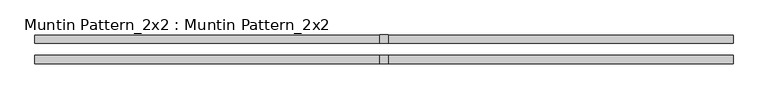
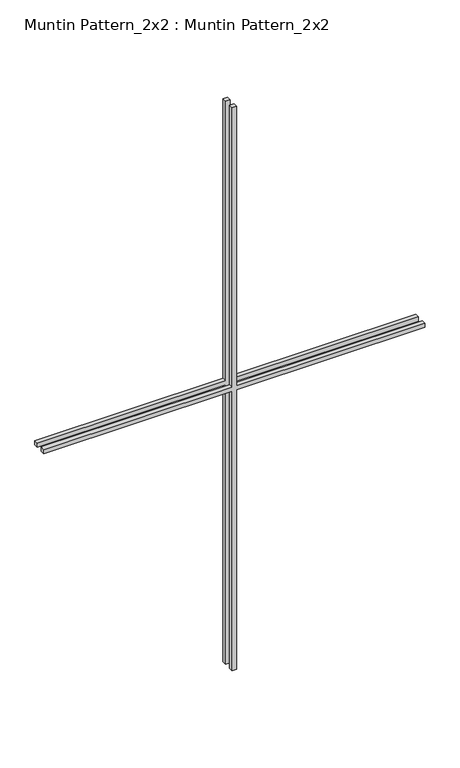
"""IFC4 building model written with IfcOpenShell, lengths in millimetres: proxy geometry, Muntin Pattern_2x2 : Muntin Pattern_2x2."""

from ifc_helpers import new_model, si_unit, frame, origin, place, context, project, spatial, polyline, outline, extrude, source, transform, mapped, element, save


def muntin_pattern_2x2_muntin_pattern_2x2_bb8d4d84(model_context):
    return source(origin(), model_context, "Body", "SweptSolid", [
        extrude(outline(polyline([(850.9, -6.35), (850.9, -541.3375), (838.2, -541.3375), (838.2, -6.35), (0.0, -6.35), (0.0, 6.35), (838.2, 6.35), (838.2, 541.3375), (850.9, 541.3375), (850.9, 6.35), (1689.1, 6.35), (1689.1, -6.35), (850.9, -6.35)])), frame((0.0, 9.525, 0.0), z_axis=(0.0, 1.0, 0.0), x_axis=(0.0, 0.0, 1.0)), (0.0, 0.0, 1.0), 12.7),
        extrude(outline(polyline([(850.9, -6.35), (850.9, -541.3375), (838.2, -541.3375), (838.2, -6.35), (0.0, -6.35), (0.0, 6.35), (838.2, 6.35), (838.2, 541.3375), (850.9, 541.3375), (850.9, 6.35), (1689.1, 6.35), (1689.1, -6.35), (850.9, -6.35)])), frame((0.0, -22.225, 0.0), z_axis=(0.0, 1.0, 0.0), x_axis=(0.0, 0.0, 1.0)), (0.0, 0.0, 1.0), 12.7),
    ])


if __name__ == "__main__":
    model = new_model("IFC4")
    model_context = context("Model", 3, world=origin())
    ifc_project = project(units=[si_unit("LENGTHUNIT", "METRE", prefix="MILLI")], contexts=[model_context])
    site = spatial("IfcSite", under=ifc_project)
    building = spatial("IfcBuilding", under=site)
    placement = place(None, origin())
    muntin_pattern_2x2_muntin_pattern_2x2_shape = muntin_pattern_2x2_muntin_pattern_2x2_bb8d4d84(model_context)
    element("IfcBuildingElementProxy", 1, Name="Muntin Pattern_2x2 : Muntin Pattern_2x2", ObjectType="Muntin Pattern_2x2 : Muntin Pattern_2x2", at=placement, inside=building, context=model_context, shape_type="MappedRepresentation", body=[
        mapped(muntin_pattern_2x2_muntin_pattern_2x2_shape, transform((0.0, 0.0, 0.0), x_axis=(1.0, 0.0, 0.0), y_axis=(0.0, 1.0, 0.0), z_axis=(0.0, 0.0, 1.0))),
    ])
    save(model, "model.ifc")

# Revit data of these elements
# Type "Muntin Pattern_2x2 : Muntin Pattern_2x2"
#   Width [instance default] = 4' - 0"
#   Thickness = 0' - 0 1/2"
#   Height [instance default] = 4' - 0"
#   Distance = 0' - 0 3/4"
#   Interior Material [instance default] = none
#   Exterior Material [instance default] = none
#   Default Elevation = 0
# Element 1 (IfcBuildingElementProxy, "Muntin Pattern_2x2 : Muntin Pattern_2x2")
#   Width = 3' - 6 5/8"
#   Height = 5' - 6 1/2"
#   Interior Material = Wood - Stained
#   Exterior Material = Clad - White
#   Materials on its faces: "Clad - White", "Wood - Stained"
# Materials
#   "Clad - White": class "Wood", colour RGB 242 242 238, transparency 0, Cost = 0
#   "Wood - Stained": class "Wood", colour RGB 224 178 126, transparency 0, Cost = 0
